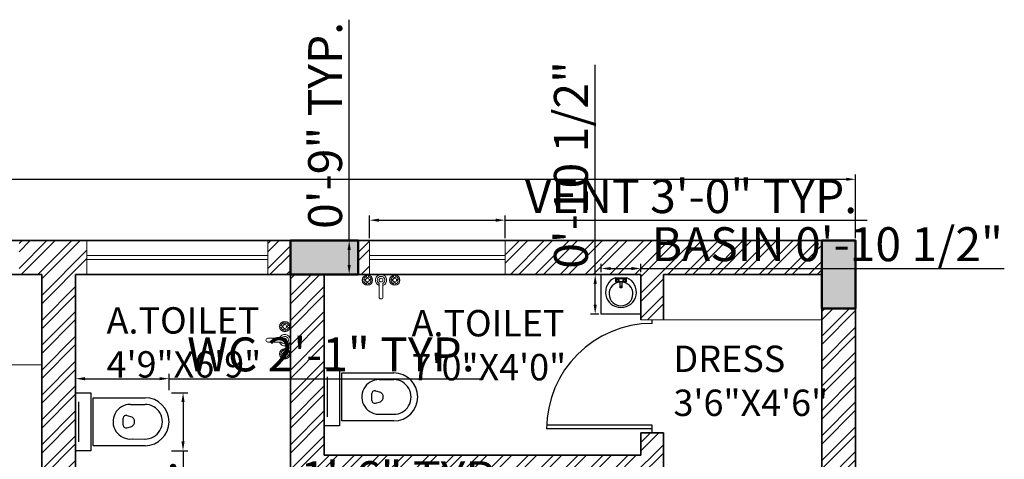
# Model space of a CAD drawing. Units: inches. Extents: x 4153 to 5577, y 785 to 1503.
# Tile 5 of 11: x 4480 to 4741, y 1386 to 1503. Entities that reach past the tile are written whole.
import ezdxf

# ---------------------------------------------------------------- set-up
doc = ezdxf.new("R2010")
doc.units = ezdxf.units.IN
for name, color, linetype, lineweight in [('A-ANNO-DIMS', 2, 'Continuous', 18), ('A-AREA-IDEN', 7, 'Continuous', 25), ('A-COLS', 7, 'Continuous', 50), ('A-DOOR', 3, 'Continuous', 25), ('A-FLOR-CASE', 32, 'Continuous', 18), ('A-GLAZ', 4, 'Continuous', 18), ('A-WALL', 7, 'Continuous', 35), ('Сантехника', 7, 'Continuous', 18)]:
    doc.layers.add(name, color=color, linetype=linetype, lineweight=lineweight)
doc.layers.add('A-WALL-PATT', color=251, linetype='Continuous', lineweight=13, true_color=0x636466)
doc.layers.add('SANTEH', color=7, linetype='Continuous')
doc.styles.get("Standard").update_dxf_attribs({"font": 'arial.ttf'})
doc.dimstyles.new('ISO-25', dxfattribs={"dimtxt": 9, "dimasz": 2.5, "dimexe": 1.25, "dimexo": 0.625, "dimtad": 1, "dimlunit": 3, "dimtxsty": 'Standard', "dimcen": 2.5, "dimadec": 0, "dimazin": 0, "dimtfac": 1, "dimtmove": 0, "dimatfit": 3, "dimfxl": 1, "dimarcsym": 0})

# ---------------------------------------------------------------- blocks, each defined once
blk = doc.blocks.new('D2')
for p, q in [((1, 0), (1, 28)), ((2, 0), (2, 27.98)), ((0, 0), (2, 0)), ((29, 0), (30, 0))]:
    blk.add_line(p, q)
at = {"ltscale": 0.5}
blk.add_arc((1, 0), 28, 0, 90, dxfattribs=at)
blk = doc.blocks.new('Faucet - Bathroom top')
for p, q in [((-4.107, 0.125), (-4.375, 0.125)), ((-3.75, 0.4788), (-3.75, 0.75)), ((-3.5, 0.482), (-3.5, 0.75)), ((-3.1461, 0.125), (-2.875, 0.125)), ((3.143, 0.125), (2.875, 0.125)), ((3.5, 0.4788), (3.5, 0.75)), ((3.75, 0.482), (3.75, 0.75)), ((4.1039, 0.125), (4.375, 0.125)), ((-4.1039, -0.125), (-4.375, -0.125)), ((-3.75, -0.4821), (-3.75, -0.75)), ((-3.5, -0.4789), (-3.5, -0.75)), ((-3.143, -0.125), (-2.875, -0.125)), ((-0.5, -0.8639), (-0.5, -4.5)), ((0.5, -4.5), (0.5, -0.8631)), ((3.1461, -0.125), (2.875, -0.125)), ((3.5, -0.4821), (3.5, -0.75)), ((3.75, -0.4789), (3.75, -0.75)), ((4.107, -0.125), (4.375, -0.125))]:
    blk.add_line(p, q)
for centre, radius in [((-3.625, 0), 1.375), ((-4.625, 0), 0.2795), ((-3.625, 0), 0.5), ((-3.625, 1), 0.2795), ((-2.625, 0), 0.2795), ((0, 0), 0.5), ((3.625, 0), 1.375), ((2.625, 0), 0.2795), ((3.625, 0), 0.5), ((3.625, 1), 0.2795), ((4.625, 0), 0.2795), ((-3.625, -1), 0.2795), ((3.625, -1), 0.2795)]:
    blk.add_circle(centre, radius)
for centre, radius, start, end in [((-3.625, 0), 1, 105.2407, 164.2093), ((-3.625, 0), 1, 16.44125, 74.07887), ((0, 0), 1.5, 289.6514, 250.3603), ((0, 0), 1, 300.3431, 239.7554), ((3.625, 0), 1, 106.12, 164.0884), ((3.625, 0), 1, 16.23422, 73.90469), ((-3.625, 0), 1, 196.2342, 253.9047), ((-3.625, 0), 1, 286.12, 344.0884), ((3.625, 0), 1, 196.4413, 254.0789), ((3.625, 0), 1, 285.2407, 344.2093), ((0, -4.5), 0.5, 180, 0)]:
    blk.add_arc(centre, radius, start, end)
blk = doc.blocks.new('y3')
at = {"layer": 'SANTEH', "ltscale": 5}
for p, q in [((37.5, 130.7), (37.5, 520.7)), ((87.5, 410.7), (87.5, 520.7)), ((346.6, 426.1), (347.5, 520.7)), ((397.5, 520.7), (397.5, 130.7)), ((171.9, 384.5), (181.1, 421.3)), ((263.1, 384.5), (253.9, 421.3)), ((244.3, 357.8), (190.7, 357.8)), ((397.5, 130.7), (37.5, 130.7)), ((67.5, 20.7), (367.5, 20.7))]:
    blk.add_line(p, q, dxfattribs=at)
blk.add_lwpolyline([(0, 115), (435, 115), (435, 0), (0, 0), (0, 115)], dxfattribs=at)
for centre, radius, start, end in [((217.5, 520.7), 180, 0, 180), ((217.5, 520.7), 130, 359.15795, 180), ((217.5, 410.7), 130, 180, 5.98548), ((190.7, 377.8), 20, 160.50385, 270), ((217.5, 399.9), 42.2, 30.52342, 149.47658), ((244.3, 377.8), 20, 270, 19.49615)]:
    blk.add_arc(centre, radius, start, end, dxfattribs=at)
blk = doc.blocks.new('r11')
at = {"layer": 'SANTEH', "ltscale": 5}
for p, q in [((0, 0), (600, 0)), ((0, -600), (0, 0)), ((600, 0), (600, -600)), ((210, -50), (390, -50)), ((210, -50), (210, -50)), ((224, -63), (376, -63)), ((224, -113), (224, -63)), ((376, -113), (224, -113)), ((233, -79), (249, -69)), ((233, -98), (233, -79)), ((249, -107), (233, -98)), ((249, -69), (266, -79)), ((266, -98), (249, -107)), ((266, -79), (266, -98)), ((288, -202), (288, -113)), ((312, -113), (312, -202)), ((334, -79), (351, -69)), ((334, -98), (334, -79)), ((351, -107), (334, -98)), ((351, -69), (367, -79)), ((367, -98), (351, -107)), ((367, -79), (367, -98)), ((376, -63), (376, -113)), ((312, -184), (288, -184)), ((312, -202), (288, -202)), ((600, -600), (0, -600))]:
    blk.add_line(p, q, dxfattribs=at)
for centre, radius, start, end in [((300, -266), 234, 112.5, 67.5), ((300, -293), 180, 93.8183, 86.1817)]:
    blk.add_arc(centre, radius, start, end, dxfattribs=at)
blk = doc.blocks.new('*D21')
at = {"layer": 'A-ANNO-DIMS', "color": 0, "lineweight": -2, "transparency": 16777216}
for p, q in [((4194.93, 1445.11), (4194.93, 1461.99)), ((4197.43, 1460.74), (4699.43, 1460.74)), ((4701.93, 1445.11), (4701.93, 1461.99))]:
    blk.add_line(p, q, dxfattribs=at)
at = {"layer": 'A-ANNO-DIMS', "color": 0, "transparency": 16777216}
for points in [[(4197.43, 1461.16), (4197.43, 1460.33), (4194.93, 1460.74)], [(4699.43, 1461.16), (4699.43, 1460.33), (4701.93, 1460.74)]]:
    blk.add_solid(points, dxfattribs=at)
at = {"layer": 'Defpoints', "color": 0, "transparency": 16777216}
for p in [(4701.93, 1460.74), (4194.93, 1444.49), (4701.93, 1444.49)]:
    blk.add_point(p, dxfattribs=at)
at = {"layer": 'A-ANNO-DIMS', "color": 0, "transparency": 16777216, "insert": (4448.43, 1465.97), "char_height": 9, "attachment_point": 5}
blk.add_mtext('42\'-3"', dxfattribs=at)
blk = doc.blocks.new('VENT-WINDOW-48IN')
for p, q in [((0, 9), (0, 0)), ((48, 9), (48, 0)), ((0, 5), (48, 5)), ((0, 4), (48, 4))]:
    blk.add_line(p, q)
blk = doc.blocks.new('VENT-WINDOW-36IN')
for p, q in [((0, 9), (0, 0)), ((36, 9), (36, 0)), ((0, 5), (36, 5)), ((0, 4), (36, 4))]:
    blk.add_line(p, q)
blk = doc.blocks.new('COL-9X18IN')
at = {"transparency": 33554687}
h = blk.add_hatch(color=256, dxfattribs=at)
h.dxf.hatch_style = 1
h.paths.add_polyline_path([(9, 18), (0, 18), (0, 0), (9, 0)])
blk.add_lwpolyline([(0, 18), (9, 18), (9, 0), (0, 0)], close=True)
blk = doc.blocks.new('*D108')
at = {"layer": 'A-ANNO-DIMS', "color": 0, "lineweight": -2, "transparency": 16777216}
for p, q in [((4572.93, 1445.11), (4572.93, 1451.14)), ((4608.93, 1445.11), (4608.93, 1451.14)), ((4575.43, 1449.89), (4606.43, 1449.89)), ((4608.93, 1449.89), (4705.03, 1449.89))]:
    blk.add_line(p, q, dxfattribs=at)
at = {"layer": 'A-ANNO-DIMS', "color": 0, "transparency": 16777216}
for points in [[(4575.43, 1450.31), (4575.43, 1449.47), (4572.93, 1449.89)], [(4606.43, 1450.31), (4606.43, 1449.47), (4608.93, 1449.89)]]:
    blk.add_solid(points, dxfattribs=at)
at = {"layer": 'Defpoints', "color": 0, "transparency": 16777216}
for p in [(4608.93, 1449.89), (4572.93, 1444.49), (4608.93, 1444.49)]:
    blk.add_point(p, dxfattribs=at)
at = {"layer": 'A-ANNO-DIMS', "color": 0, "transparency": 16777216, "insert": (4658.23, 1455.11), "char_height": 9, "attachment_point": 5}
blk.add_mtext('VENT 3\'-0" TYP.', dxfattribs=at)
blk = doc.blocks.new('*D109')
at = {"layer": 'A-ANNO-DIMS', "color": 0, "lineweight": -2, "transparency": 16777216}
for p, q in [((4567.53, 1444.49), (4567.53, 1503.1)), ((4572.3, 1444.49), (4566.28, 1444.49)), ((4567.53, 1437.99), (4567.53, 1441.99)), ((4572.3, 1435.49), (4566.28, 1435.49))]:
    blk.add_line(p, q, dxfattribs=at)
at = {"layer": 'A-ANNO-DIMS', "color": 0, "transparency": 16777216}
for points in [[(4567.11, 1441.99), (4567.94, 1441.99), (4567.53, 1444.49)], [(4567.11, 1437.99), (4567.94, 1437.99), (4567.53, 1435.49)]]:
    blk.add_solid(points, dxfattribs=at)
at = {"layer": 'Defpoints', "color": 0, "transparency": 16777216}
for p in [(4567.53, 1444.49), (4572.93, 1444.49), (4572.93, 1435.49)]:
    blk.add_point(p, dxfattribs=at)
at = {"layer": 'A-ANNO-DIMS', "color": 0, "transparency": 16777216, "insert": (4562.31, 1475.04), "char_height": 9, "attachment_point": 5, "rotation": 90}
blk.add_mtext('0\'-9" TYP.', dxfattribs=at)
blk = doc.blocks.new('*D118')
at = {"layer": 'A-ANNO-DIMS', "color": 0, "lineweight": -2, "transparency": 16777216}
for p, q in [((4494.93, 1404.74), (4494.93, 1409.08)), ((4519.72, 1404.74), (4519.72, 1409.08)), ((4497.43, 1407.83), (4517.22, 1407.83)), ((4519.72, 1407.83), (4603.14, 1407.83))]:
    blk.add_line(p, q, dxfattribs=at)
at = {"layer": 'A-ANNO-DIMS', "color": 0, "transparency": 16777216}
for points in [[(4497.43, 1408.25), (4497.43, 1407.41), (4494.93, 1407.83)], [(4517.22, 1408.25), (4517.22, 1407.41), (4519.72, 1407.83)]]:
    blk.add_solid(points, dxfattribs=at)
at = {"layer": 'Defpoints', "color": 0, "transparency": 16777216}
for p in [(4519.72, 1407.83), (4494.93, 1404.11), (4519.72, 1404.11)]:
    blk.add_point(p, dxfattribs=at)
at = {"layer": 'A-ANNO-DIMS', "color": 0, "transparency": 16777216, "insert": (4562.68, 1413.11), "char_height": 9, "attachment_point": 5}
blk.add_mtext('WC 2\'-1" TYP.', dxfattribs=at)
blk = doc.blocks.new('*D119')
at = {"layer": 'A-ANNO-DIMS', "color": 0, "lineweight": -2, "transparency": 16777216}
for p, q in [((4520.35, 1404.11), (4524.69, 1404.11)), ((4523.44, 1401.61), (4523.44, 1391.22)), ((4520.35, 1388.72), (4524.69, 1388.72)), ((4523.44, 1388.72), (4523.44, 1309.99))]:
    blk.add_line(p, q, dxfattribs=at)
at = {"layer": 'A-ANNO-DIMS', "color": 0, "transparency": 16777216}
for points in [[(4523.02, 1401.61), (4523.86, 1401.61), (4523.44, 1404.11)], [(4523.02, 1391.22), (4523.86, 1391.22), (4523.44, 1388.72)]]:
    blk.add_solid(points, dxfattribs=at)
at = {"layer": 'Defpoints', "color": 0, "transparency": 16777216}
for p in [(4519.72, 1404.11), (4519.72, 1388.72), (4523.44, 1388.72)]:
    blk.add_point(p, dxfattribs=at)
at = {"layer": 'A-ANNO-DIMS', "color": 0, "transparency": 16777216, "insert": (4518.16, 1348.1), "char_height": 9, "attachment_point": 5, "rotation": 90}
blk.add_mtext('1\'-3 1/2" TYP.', dxfattribs=at)
blk = doc.blocks.new('*D121')
at = {"layer": 'A-ANNO-DIMS', "color": 0, "lineweight": -2, "transparency": 16777216}
for p, q in [((4534.06, 1372.98), (4534.06, 1376.29)), ((4536.56, 1375.04), (4549.43, 1375.04)), ((4551.93, 1372.98), (4551.93, 1376.29)), ((4551.93, 1375.04), (4609.69, 1375.04))]:
    blk.add_line(p, q, dxfattribs=at)
at = {"layer": 'A-ANNO-DIMS', "color": 0, "transparency": 16777216}
for points in [[(4536.56, 1375.45), (4536.56, 1374.62), (4534.06, 1375.04)], [(4549.43, 1375.45), (4549.43, 1374.62), (4551.93, 1375.04)]]:
    blk.add_solid(points, dxfattribs=at)
at = {"layer": 'Defpoints', "color": 0, "transparency": 16777216}
for p in [(4551.93, 1375.04), (4534.06, 1372.36), (4551.93, 1372.36)]:
    blk.add_point(p, dxfattribs=at)
at = {"layer": 'A-ANNO-DIMS', "color": 0, "transparency": 16777216, "insert": (4582.06, 1380.26), "char_height": 9, "attachment_point": 5}
blk.add_mtext('1\'-6" TYP.', dxfattribs=at)
blk = doc.blocks.new('*D122')
at = {"layer": 'A-ANNO-DIMS', "color": 0, "lineweight": -2, "transparency": 16777216}
for p, q in [((4634.4, 1436.11), (4634.4, 1438.32)), ((4644.93, 1436.11), (4644.93, 1438.32)), ((4636.9, 1437.07), (4642.43, 1437.07)), ((4644.93, 1437.07), (4741.39, 1437.07))]:
    blk.add_line(p, q, dxfattribs=at)
at = {"layer": 'A-ANNO-DIMS', "color": 0, "transparency": 16777216}
for points in [[(4636.9, 1437.48), (4636.9, 1436.65), (4634.4, 1437.07)], [(4642.43, 1437.48), (4642.43, 1436.65), (4644.93, 1437.07)]]:
    blk.add_solid(points, dxfattribs=at)
at = {"layer": 'Defpoints', "color": 0, "transparency": 16777216}
for p in [(4634.4, 1435.49), (4644.93, 1437.07), (4644.93, 1435.49)]:
    blk.add_point(p, dxfattribs=at)
at = {"layer": 'A-ANNO-DIMS', "color": 0, "transparency": 16777216, "insert": (4694.41, 1442.35), "char_height": 9, "attachment_point": 5}
blk.add_mtext('BASIN 0\'-10 1/2"', dxfattribs=at)
blk = doc.blocks.new('*D123')
at = {"layer": 'A-ANNO-DIMS', "color": 0, "lineweight": -2, "transparency": 16777216}
for p, q in [((4632.82, 1435.49), (4632.82, 1491.13)), ((4633.78, 1435.49), (4631.57, 1435.49)), ((4632.82, 1427.46), (4632.82, 1432.99)), ((4633.78, 1424.96), (4631.57, 1424.96))]:
    blk.add_line(p, q, dxfattribs=at)
at = {"layer": 'A-ANNO-DIMS', "color": 0, "transparency": 16777216}
for points in [[(4632.4, 1432.99), (4633.24, 1432.99), (4632.82, 1435.49)], [(4632.4, 1427.46), (4633.24, 1427.46), (4632.82, 1424.96)]]:
    blk.add_solid(points, dxfattribs=at)
at = {"layer": 'Defpoints', "color": 0, "transparency": 16777216}
for p in [(4632.82, 1435.49), (4634.4, 1435.49), (4634.4, 1424.96)]:
    blk.add_point(p, dxfattribs=at)
at = {"layer": 'A-ANNO-DIMS', "color": 0, "transparency": 16777216, "insert": (4627.54, 1464.56), "char_height": 9, "attachment_point": 5, "rotation": 90}
blk.add_mtext('0\'-10 1/2"', dxfattribs=at)

msp = doc.modelspace()

# ---------------------------------------------------------------- hatches: boundary and pattern name
at = {"layer": 'A-WALL-PATT', "transparency": 33554687}
h = msp.add_hatch(dxfattribs=at)
h.set_pattern_fill('ANSI32', color=256, scale=0.49)
h.paths.add_polyline_path([(4344.927, 1138.488), (4281.927, 1138.488), (4281.927, 1234.488), (4296.927, 1234.488), (4296.927, 1243.488), (4269.927, 1243.488), (4269.927, 1234.488), (4275.927, 1234.488), (4275.927, 1138.488), (4203.927, 1138.488), (4203.927, 1168.488), (4194.927, 1168.488), (4194.927, 1088.988), (4203.927, 1088.988), (4203.927, 1129.488), (4338.927, 1129.488), (4338.927, 1105.488), (4344.927, 1105.488)])
h.paths.add_polyline_path([(4203.927, 1040.988), (4194.927, 1040.988), (4194.927, 1009.488), (4203.927, 1009.488)])
h.paths.add_polyline_path([(4278.927, 1000.488), (4203.927, 1000.488), (4203.927, 991.488), (4278.927, 991.488)])
h.paths.add_polyline_path([(4203.927, 991.488), (4194.927, 991.488), (4194.927, 910.488), (4203.927, 910.488)])
h.paths.add_polyline_path([(4335.927, 907.488), (4203.927, 907.488), (4203.927, 901.488), (4335.927, 901.488)])
h.paths.add_polyline_path([(4344.927, 1057.488), (4338.927, 1057.488), (4338.927, 1000.488), (4344.927, 1000.488)])
h.paths.add_polyline_path([(4335.927, 1000.488), (4326.927, 1000.488), (4326.927, 991.488), (4335.927, 991.488)])
h.paths.add_polyline_path([(4368.927, 1000.488), (4344.927, 1000.488), (4344.927, 991.488), (4368.927, 991.488)])
h.paths.add_polyline_path([(4440.927, 1000.488), (4416.927, 1000.488), (4416.927, 991.488), (4440.927, 991.488)])
h.paths.add_polyline_path([(4449.927, 1120.488), (4440.927, 1120.488), (4440.927, 1000.488), (4449.927, 1000.488)])
h.paths.add_polyline_path([(4473.927, 1000.488), (4458.927, 1000.488), (4458.927, 991.488), (4473.927, 991.488)])
h.paths.add_polyline_path([(4638.927, 1000.488), (4545.927, 1000.488), (4545.927, 991.488), (4638.927, 991.488)])
h.paths.add_polyline_path([(4701.927, 1036.488), (4692.927, 1036.488), (4692.927, 1009.488), (4701.927, 1009.488)])
h.paths.add_polyline_path([(4692.927, 1000.488), (4686.927, 1000.488), (4686.927, 991.488), (4692.927, 991.488)])
h.paths.add_polyline_path([(4701.927, 1132.488), (4692.927, 1132.488), (4692.927, 1108.488), (4701.927, 1108.488)])
h.paths.add_polyline_path([(4701.927, 1225.488), (4692.927, 1225.488), (4692.927, 1204.488), (4701.927, 1204.488)])
h.paths.add_polyline_path([(4650.927, 1243.488), (4560.927, 1243.488), (4560.927, 1265.228), (4560.927, 1381.488), (4650.927, 1381.488), (4650.927, 1393.488), (4644.927, 1393.488), (4644.927, 1387.488), (4560.927, 1387.488), (4560.927, 1435.488), (4551.927, 1435.488), (4551.927, 1354.488), (4530.927, 1354.488), (4530.927, 1348.488), (4551.927, 1348.488), (4551.927, 1309.488), (4485.927, 1309.488), (4485.927, 1234.488), (4505.427, 1234.488), (4505.427, 1243.488), (4494.927, 1243.488), (4494.927, 1303.488), (4551.927, 1303.488), (4551.927, 1243.488), (4541.427, 1243.488), (4541.427, 1234.488), (4650.927, 1234.488)])
h.paths.add_polyline_path([(4701.927, 1426.488), (4692.927, 1426.488), (4692.927, 1357.488), (4701.927, 1357.488)])
h.paths.add_polyline_path([(4701.927, 1309.488), (4692.927, 1309.488), (4692.927, 1243.488), (4701.927, 1243.488)])
h.paths.add_polyline_path([(4692.927, 1444.488), (4608.927, 1444.488), (4608.927, 1435.488), (4644.927, 1435.488), (4644.927, 1423.488), (4650.927, 1423.488), (4650.927, 1435.488), (4692.927, 1435.488)])
h.paths.add_polyline_path([(4497.927, 1444.488), (4479.927, 1444.488), (4479.927, 1435.488), (4485.927, 1435.488), (4485.927, 1348.488), (4500.927, 1348.488), (4500.927, 1354.488), (4494.927, 1354.488), (4494.927, 1435.488), (4497.927, 1435.488)])
h.paths.add_polyline_path([(4551.927, 1444.488), (4545.927, 1444.488), (4545.927, 1435.488), (4551.927, 1435.488)])
h.paths.add_polyline_path([(4572.927, 1444.488), (4569.927, 1444.488), (4569.927, 1435.488), (4572.927, 1435.488)])
h.paths.add_polyline_path([(4431.927, 1444.488), (4356.927, 1444.488), (4356.927, 1435.488), (4431.927, 1435.488)])
h.paths.add_polyline_path([(4284.927, 1444.488), (4203.927, 1444.488), (4203.927, 1435.488), (4284.927, 1435.488)])
h.paths.add_polyline_path([(4203.927, 1426.488), (4194.927, 1426.488), (4194.927, 1293.488), (4203.927, 1293.488), (4203.927, 1295.242)])
h.paths.add_polyline_path([(4347.927, 1435.488), (4338.927, 1435.488), (4338.927, 1243.488), (4332.927, 1243.488), (4332.927, 1234.488), (4431.927, 1234.488), (4431.927, 1243.488), (4347.927, 1243.488)])
h.paths.add_polyline_path([(4239.927, 1243.488), (4203.927, 1243.488), (4203.927, 1234.488), (4239.927, 1234.488)], flags=17)
h.paths.add_polyline_path([(4203.927, 1225.488), (4194.927, 1225.488), (4194.927, 1198.488), (4203.927, 1198.488)], flags=17)

# ---------------------------------------------------------------- linework, layer by layer
at = {"layer": 'A-FLOR-CASE'}
for p, q in [((4644.927, 1423.488), (4692.927, 1423.488)), ((4347.927, 1411.488), (4485.927, 1411.488))]:
    msp.add_line(p, q, dxfattribs=at)
at = {"layer": 'A-WALL'}
for p, q in [((4194.927, 1444.488), (4701.927, 1444.488)), ((4701.927, 1444.488), (4701.927, 901.488)), ((4347.927, 1435.488), (4485.927, 1435.488)), ((4485.927, 1348.488), (4485.927, 1435.488)), ((4494.927, 1435.488), (4551.927, 1435.488)), ((4494.927, 1354.488), (4494.927, 1435.488)), ((4551.927, 1354.488), (4551.927, 1435.488)), ((4560.927, 1435.488), (4644.927, 1435.488)), ((4560.927, 1387.488), (4560.927, 1435.488)), ((4644.927, 1423.488), (4644.927, 1435.488)), ((4650.927, 1435.488), (4692.927, 1435.488)), ((4650.927, 1423.488), (4650.927, 1435.488)), ((4692.927, 1435.488), (4692.927, 1243.488)), ((4644.927, 1387.488), (4644.927, 1393.488)), ((4644.927, 1393.488), (4650.927, 1393.488)), ((4650.927, 1357.488), (4650.927, 1393.488)), ((4560.927, 1387.488), (4644.927, 1387.488))]:
    msp.add_line(p, q, dxfattribs=at)

# ---------------------------------------------------------------- block references
at = {"layer": 'A-COLS', "rotation": 270.0000000000056}
msp.add_blockref('COL-9X18IN', (4551.927, 1444.488), dxfattribs=at)
at = {"layer": 'A-COLS'}
msp.add_blockref('COL-9X18IN', (4692.927, 1426.488), dxfattribs=at)
at = {"layer": 'A-DOOR', "rotation": 90}
msp.add_blockref('D2', (4647.927, 1393.488), dxfattribs=at)
at = {"layer": 'A-GLAZ'}
for name, p in [('VENT-WINDOW-48IN', (4497.927, 1435.488)), ('VENT-WINDOW-36IN', (4572.927, 1435.488))]:
    msp.add_blockref(name, p, dxfattribs=at)
at = {"layer": 'Сантехника', "xscale": -1}
msp.add_blockref('Faucet - Bathroom top', (4575.991, 1433.988), dxfattribs=at)
at = {"layer": 'Сантехника', "xscale": 0.0175454563869893, "yscale": 0.0175454563869893, "zscale": 0.0175454563869893}
msp.add_blockref('r11', (4634.4, 1435.488), dxfattribs=at)
at = {"layer": 'Сантехника', "xscale": -1, "rotation": 270}
msp.add_blockref('Faucet - Bathroom top', (4550.427, 1418.048), dxfattribs=at)
at = {"layer": 'Сантехника', "xscale": 0.0353848906415677, "yscale": 0.0353848906415677, "zscale": 0.0353848906415677, "rotation": 270}
for p in [(4560.927, 1410.677), (4494.927, 1404.112)]:
    msp.add_blockref('y3', p, dxfattribs=at)

# ---------------------------------------------------------------- texts
at = {"layer": 'A-AREA-IDEN', "char_height": 7, "attachment_point": 1}
for s, heights, insert in [('{\\fTimes New Roman|b0|i0|c0|p18;A.TOILET\\P4\'9"X6\'9"}', [18.808], (4503.155, 1426.791)), ('{\\fTimes New Roman|b0|i0|c0|p18;A.TOILET\\P7\'0"X4\'0"}', [0], (4584.082, 1426.054)), ('{\\fTimes New Roman|b0|i0|c0|p18;DRESS\\P3\'6"X4\'6"}', [0], (4653.606, 1416.602))]:
    msp.add_mtext_dynamic_manual_height_columns(s, width=67.35079, gutter_width=12.5, heights=heights, dxfattribs=dict(at, insert=insert))

# ---------------------------------------------------------------- dimensions: what is measured, and where the dimension line sits
at = {"layer": 'A-ANNO-DIMS'}
for base, p1, p2, angle, picture, middle in [((4567.527, 1444.488), (4572.927, 1435.488), (4572.927, 1444.488), 90, '*D109', (4562.307, 1475.043)), ((4523.441, 1388.72), (4519.721, 1404.112), (4519.721, 1388.72), 270, '*D119', (4518.159, 1348.103))]:
    dim = msp.add_linear_dim(base=base, p1=p1, p2=p2, angle=angle, text='<> TYP.', dimstyle='ISO-25', override={"dimdec": 1, "dimlfac": 1, "dimrnd": 0, "dimzin": 1, "dimdsep": 46, "dimlunit": 4, "dimfrac": 2}, dxfattribs=at)
    dim.commit()
    dim.dimension.update_dxf_attribs({"geometry": picture, "text_midpoint": middle})
dim = msp.add_linear_dim(base=(4632.821, 1435.488), p1=(4634.4, 1424.961), p2=(4634.4, 1435.488), angle=90, dimstyle='ISO-25', override={"dimdec": 1, "dimlfac": 1, "dimrnd": 0, "dimzin": 1, "dimdsep": 46, "dimlunit": 4, "dimfrac": 2}, dxfattribs=at)
dim.commit()
dim.dimension.update_dxf_attribs({"geometry": '*D123', "text_midpoint": (4627.543, 1464.557)})
for base, p1, p2, text, picture, middle in [((4608.927, 1449.888), (4572.927, 1444.488), (4608.927, 1444.488), 'VENT <> TYP.', '*D108', (4658.228, 1455.112)), ((4644.927, 1437.067), (4634.4, 1435.488), (4644.927, 1435.488), 'BASIN <>', '*D122', (4694.409, 1442.346)), ((4519.721, 1407.831), (4494.927, 1404.112), (4519.721, 1404.112), 'WC <> TYP.', '*D118', (4562.68, 1413.11)), ((4551.927, 1375.037), (4534.059, 1372.356), (4551.927, 1372.356), '<> TYP.', '*D121', (4582.059, 1380.257))]:
    dim = msp.add_linear_dim(base=base, p1=p1, p2=p2, text=text, dimstyle='ISO-25', override={"dimdec": 1, "dimlfac": 1, "dimrnd": 0, "dimzin": 1, "dimdsep": 46, "dimlunit": 4, "dimfrac": 2}, dxfattribs=at)
    dim.commit()
    dim.dimension.update_dxf_attribs({"geometry": picture, "text_midpoint": middle})
dim = msp.add_linear_dim(base=(4701.927, 1460.744), p1=(4194.927, 1444.488), p2=(4701.927, 1444.488), dimstyle='ISO-25', override={"dimclrd": 0, "dimclre": 0, "dimclrt": 0}, dxfattribs=at)
dim.commit()
dim.dimension.update_dxf_attribs({"geometry": '*D21', "text_midpoint": (4448.427, 1465.968)})

doc.saveas('drawing.dxf')
